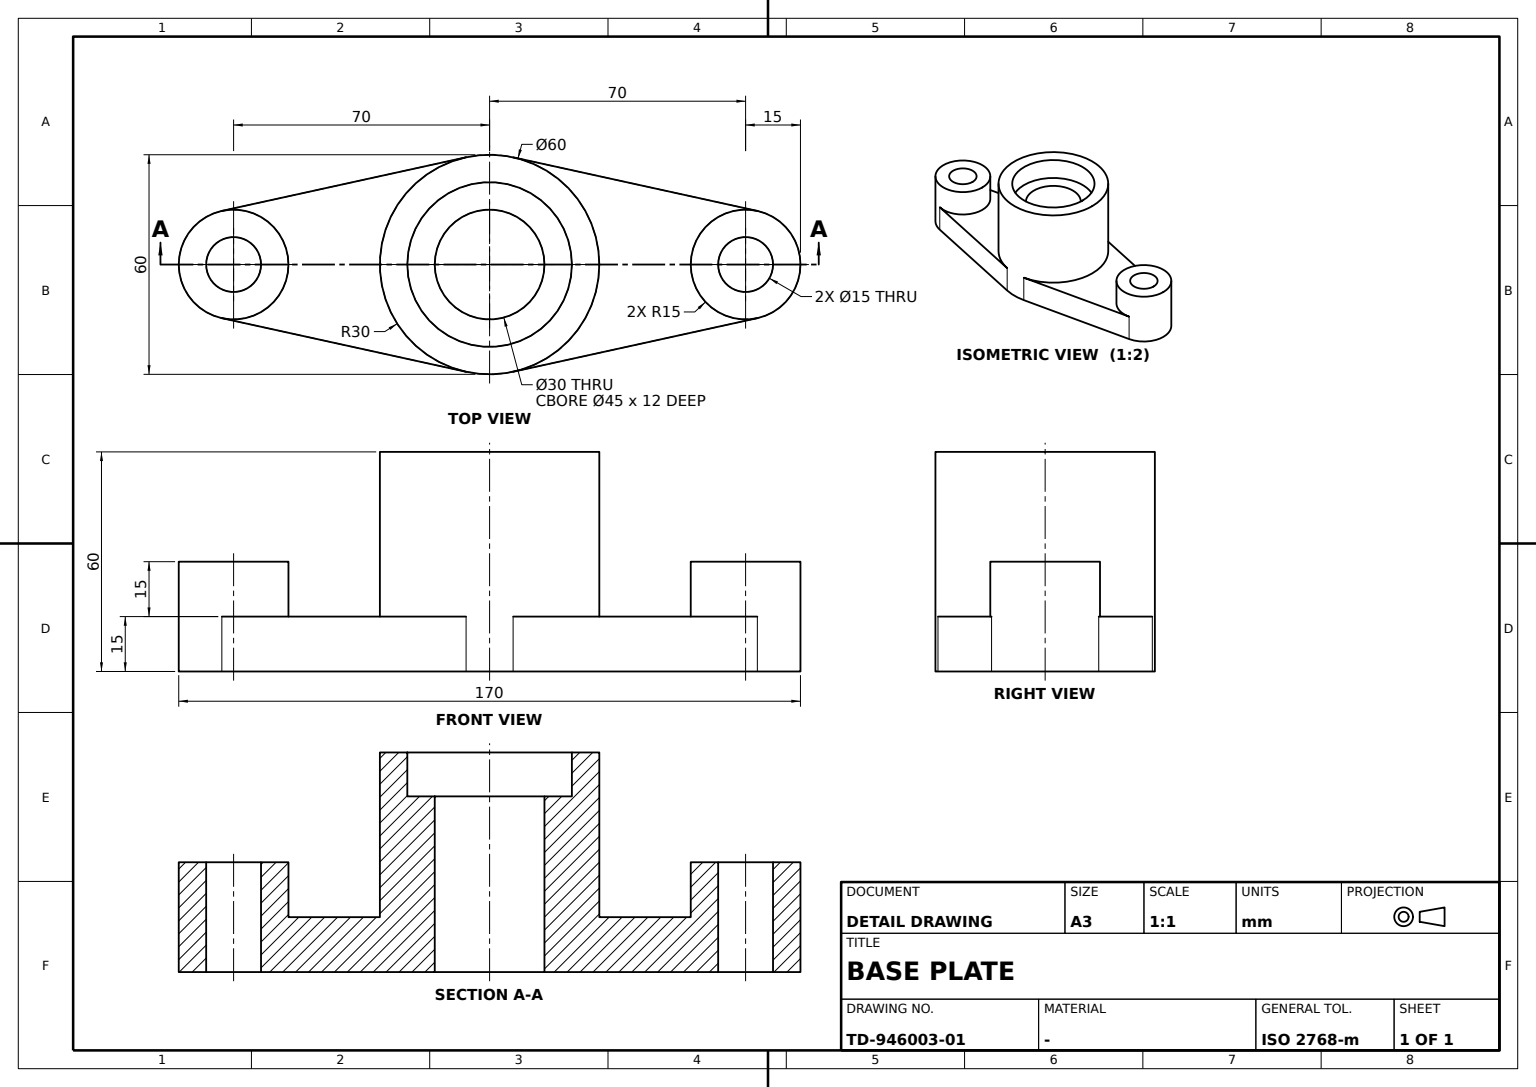
CATIA V5 part; units mm, degrees
sketch "Sketch1" plane through (0, 0, 0) normal (0, 0, 1) x (1, 0, 0)
  arc A0 (6.4286, 29.3031) -> (-6.4286, 29.3031) centre (0, 0) ccw
  arc A1 (73.2143, -14.6516) -> (73.2143, 14.6516) centre (70, 0) ccw
  point P0 (70, 0)
  arc A2 (-73.2143, -14.6516) -> (-73.2143, 14.6516) centre (-70, 0) cw
  line L0 (-73.2143, 14.6516) -> (-6.4286, 29.3031)
  line L1 (6.4286, 29.3031) -> (73.2143, 14.6516)
  point P1 (73.2143, 14.6516)
  point P2 (0, 30.7134)
  point P3 (-73.2143, 14.6516)
  point P4 (73.2143, -14.6516)
  line L2 (6.4286, -29.3031) -> (73.2143, -14.6516)
  point P5 (-73.2143, -14.6516)
  line L3 (-73.2143, -14.6516) -> (-6.4286, -29.3031)
  arc A3 (-6.4286, -29.3031) -> (6.4286, -29.3031) centre (0, 0) ccw
  dimension "radius A0" = 30
  dimension "radius A1" = 15
  dimension "distance origin P0" = 70
  constraint coincidence P0 x-axis
  constraint coincidence A0 A3
  constraint symmetry A1 A2 y-axis
  constraint symmetry P1 P4 x-axis
  constraint symmetry L1 L2 x-axis
  constraint symmetry P3 P5 x-axis
  constraint symmetry L0 L3 x-axis
  constraint tangency L0 A2
  constraint tangency L0 A0
  constraint tangency L1 A1
  constraint tangency L1 A0
extrude "Pad1" add sketch "Sketch1" along normal blind 15
sketch "Sketch2" plane through (0, 0, 0) normal (0, 0, 1) x (1, 0, 0)
  circle A0 centre (0, 0) radius 30
  dimension "radius A0" = 30
extrude "Pad2" add sketch "Sketch2" along normal blind 60
sketch "Sketch3" plane through (0, 0, 0) normal (0, 0, 1) x (1, 0, 0)
  circle A0 centre (70, 0) radius 15
  point P0 (70, 0)
  circle A1 centre (-70, 0) radius 15
  dimension "radius A0" = 15
  dimension "distance y axis P0" = 70
  constraint coincidence P0 x-axis
  constraint symmetry A0 A1 y-axis
extrude "Pad3" add sketch "Sketch3" along normal blind 30
sketch "Sketch4" plane through (0, 0, 60) normal (0, 0, 1) x (1, 0, 0)
  circle A0 centre (0, 0) radius 15
  circle A1 centre (70, 0) radius 7.5
  point P0 (70, 0)
  circle A2 centre (-70, 0) radius 7.5
  dimension "radius A0" = 15
  dimension "radius A1" = 7.5
  dimension "distance y axis P0" = 70
  constraint coincidence P0 x-axis
  constraint symmetry A1 A2 y-axis
extrude "Pocket1" cut sketch "Sketch4" against normal blind 60
sketch "Sketch5" plane through (0, 0, 60) normal (0, 0, 1) x (1, 0, 0)
  circle A0 centre (0, 0) radius 22.5
  dimension "radius A0" = 22.5
extrude "Pocket2" cut sketch "Sketch5" against normal blind 12
